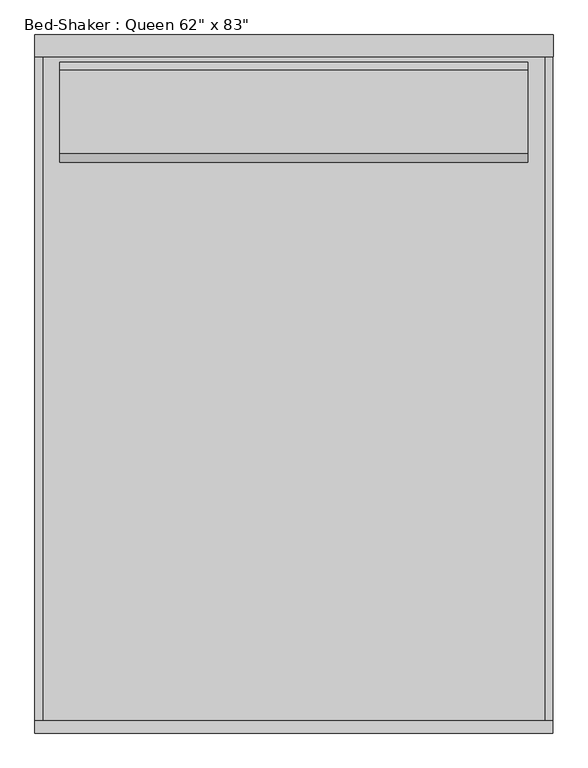
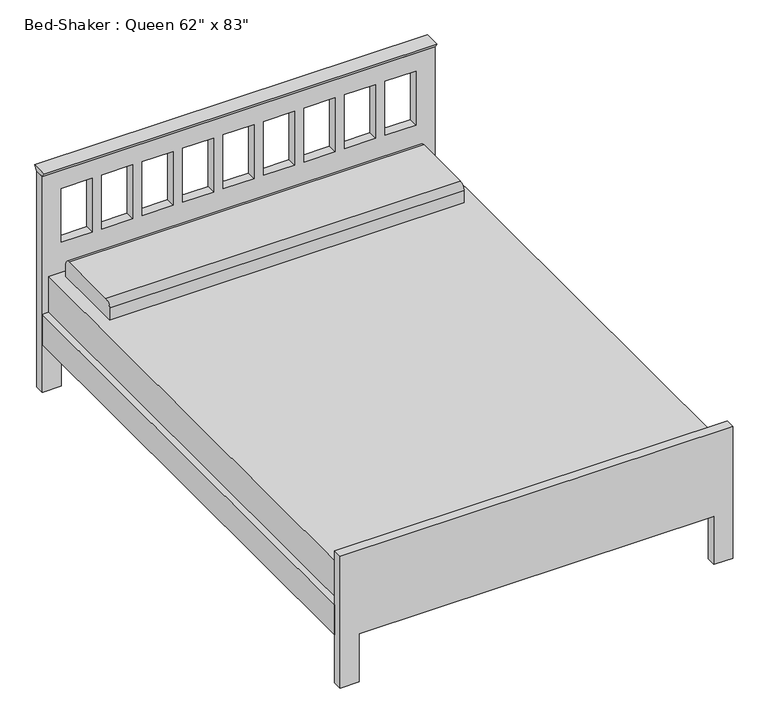
"""IFC4 building model written with IfcOpenShell, lengths in millimetres: furniture geometry."""

from ifc_helpers import new_model, si_unit, point, frame, frame_2d, origin, place, context, project, spatial, polyline, circle_curve, trimmed, segment, composite_curve, outline, extrude, source, transform, mapped, element, save


def furniture_35c09872(model_context):
    return source(origin(), model_context, "Body", "SweptSolid", [
        extrude(outline(polyline([(-38.1, 914.4), (-51.9545455, 933.45), (13.8545455, 933.45), (0.0, 914.4), (-38.1, 914.4)])), frame((-806.2365546, 0.0, 0.0), z_axis=(1.0, 0.0, 0.0), x_axis=(0.0, 1.0, 0.0)), (0.0, 0.0, 1.0), 1574.8533613),
        extrude(outline(composite_curve([segment(polyline([(-373.2486637, 482.6), (-373.2486637, 533.4)]), True, "CONTINUOUS"), segment(trimmed(circle_curve(frame_2d((-347.8486637, 533.4)), 25.4), [point((-373.2486637, 533.4))], [point((-347.8486637, 558.8))], False, "CARTESIAN"), True, "CONTINUOUS"), segment(polyline([(-347.8486637, 558.8), (-93.8486637, 558.8)]), True, "CONTINUOUS"), segment(trimmed(circle_curve(frame_2d((-93.8486637, 533.4)), 25.4), [point((-93.8486637, 558.8))], [point((-68.4486637, 533.4))], False, "CARTESIAN"), True, "CONTINUOUS"), segment(polyline([(-68.4486637, 533.4), (-68.4486637, 482.6), (-373.2486637, 482.6)]), True, "CONTINUOUS")], self_intersect=False)), frame((-730.25, 0.0, 0.0), z_axis=(1.0, 0.0, 0.0), x_axis=(0.0, 1.0, 0.0)), (0.0, 0.0, 1.0), 1422.4),
        extrude(outline(polyline([(742.95, -38.1), (742.95, -2070.1), (-781.05, -2070.1), (-781.05, -38.1), (742.95, -38.1)])), frame((0.0, 0.0, 228.6), z_axis=(0.0, 0.0, 1.0), x_axis=(1.0, 0.0, 0.0)), (0.0, 0.0, 1.0), 254.0),
        extrude(outline(polyline([(742.95, -2070.1), (742.95, -38.1), (768.35, -38.1), (768.35, -2070.1), (742.95, -2070.1)])), frame((0.0, 0.0, 203.0994861), z_axis=(0.0, 0.0, 1.0), x_axis=(1.0, 0.0, 0.0)), (0.0, 0.0, 1.0), 127.0),
        extrude(outline(polyline([(-806.45, -2070.1), (-806.45, -38.1), (-781.05, -38.1), (-781.05, -2070.1), (-806.45, -2070.1)])), frame((0.0, 0.0, 203.5755296), z_axis=(0.0, 0.0, 1.0), x_axis=(1.0, 0.0, 0.0)), (0.0, 0.0, 1.0), 127.0),
        extrude(outline(polyline([(0.0, -730.25), (203.2, -730.25), (203.2, 692.15), (0.0, 692.15), (0.0, 768.35), (558.8, 768.35), (558.8, -806.45), (0.0, -806.45), (0.0, -730.25)])), frame((0.0, -2108.2, 0.0), z_axis=(0.0, 1.0, 0.0), x_axis=(0.0, 0.0, 1.0)), (0.0, 0.0, 1.0), 38.1),
        extrude(outline(polyline([(914.4, 768.6168067), (914.4, -806.2365546), (0.0, -806.2365546), (0.0, -730.25), (203.2, -730.25), (203.2, 692.15), (0.0, 692.15), (0.0, 768.6168067), (914.4, 768.6168067)]), holes=[polyline([(838.2, -606.0722222), (609.6, -606.0722222), (609.6, -730.25), (838.2, -730.25), (838.2, -606.0722222)]), polyline([(838.2, -443.7944444), (609.6, -443.7944444), (609.6, -567.9722222), (838.2, -567.9722222), (838.2, -443.7944444)]), polyline([(838.2, -281.5166667), (609.6, -281.5166667), (609.6, -405.6944444), (838.2, -405.6944444), (838.2, -281.5166667)]), polyline([(838.2, -119.2388889), (609.6, -119.2388889), (609.6, -243.4166667), (838.2, -243.4166667), (838.2, -119.2388889)]), polyline([(838.2, 205.3166667), (609.6, 205.3166667), (609.6, 81.1388889), (838.2, 81.1388889), (838.2, 205.3166667)]), polyline([(838.2, 367.5944444), (609.6, 367.5944444), (609.6, 243.4166667), (838.2, 243.4166667), (838.2, 367.5944444)]), polyline([(838.2, 529.8722222), (609.6, 529.8722222), (609.6, 405.6944444), (838.2, 405.6944444), (838.2, 529.8722222)]), polyline([(838.2, 692.15), (609.6, 692.15), (609.6, 567.9722222), (838.2, 567.9722222), (838.2, 692.15)]), polyline([(838.2, 43.0388889), (609.6, 43.0388889), (609.6, -81.1388889), (838.2, -81.1388889), (838.2, 43.0388889)])]), frame((0.0, -38.1, 0.0), z_axis=(0.0, 1.0, 0.0), x_axis=(0.0, 0.0, 1.0)), (0.0, 0.0, 1.0), 38.1),
    ])


if __name__ == "__main__":
    model = new_model("IFC4")
    model_context = context("Model", 3, world=origin())
    ifc_project = project(units=[si_unit("LENGTHUNIT", "METRE", prefix="MILLI")], contexts=[model_context])
    site = spatial("IfcSite", under=ifc_project)
    building = spatial("IfcBuilding", under=site)
    placement = place(None, origin())
    furniture_shape = furniture_35c09872(model_context)
    element("IfcFurniture", 1, ObjectType="Bed-Shaker : Queen 62\" x 83\"", at=placement, inside=building, context=model_context, shape_type="MappedRepresentation", body=[
        mapped(furniture_shape, transform((0.0, 0.0, 0.0), x_axis=(1.0, 0.0, 0.0), y_axis=(0.0, 1.0, 0.0), z_axis=(0.0, 0.0, 1.0))),
    ])
    save(model, "model.ifc")

# Revit data of these elements
# Type "Bed-Shaker : Queen 62\" x 83\""
#   Assembly Code = "E2020200"
#   Length = 6' - 11"
#   Width = 5' - 2"
#   Frame Material = Birch
#   Mattress Material = Linen, White
#   Default Elevation = 0
# Element 1 (IfcFurniture, "Bed-Shaker : Queen 62\" x 83\"")
#   Materials on its faces: "Birch", "Linen, White"
# Materials
#   "Birch": class "Wood", colour RGB 224 178 126, transparency 0, Description = "Betula Alleghaniensis", Cost = 0
#   "Linen, White": class "Textile", colour RGB 247 247 239, transparency 0, Description = "Linen, white", Cost = 0
